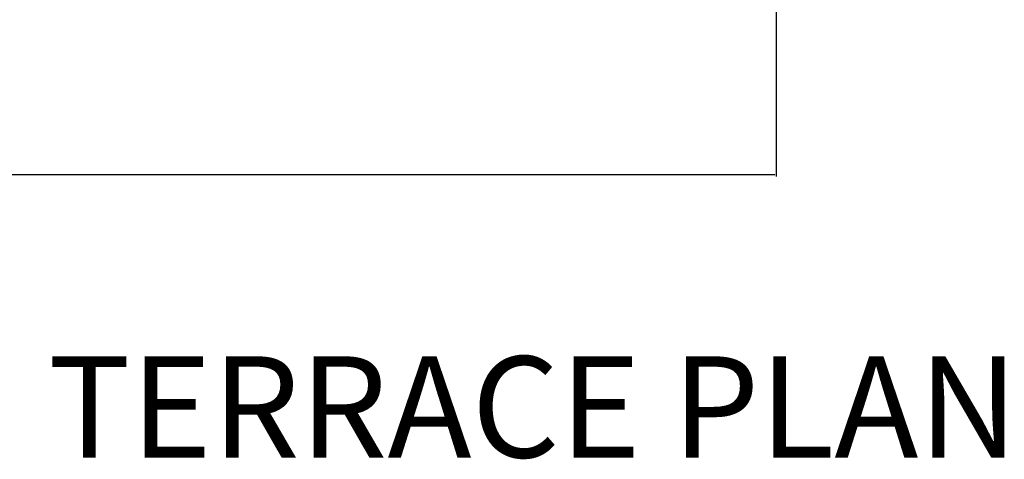
# Model space of a CAD drawing. Units: inches. Extents: x 2166 to 3588, y 1959 to 2628.
# Tile 4 of 13: x 3339 to 3455, y 1964 to 2016. Entities that reach past the tile are written whole.
import ezdxf

# ---------------------------------------------------------------- set-up
doc = ezdxf.new("R2010")
doc.units = ezdxf.units.IN
doc.layers.add('A-ANNO-DIMS', color=2, linetype='Continuous', lineweight=18)
doc.layers.add('A-ANNO-TITL', color=170, linetype='Continuous', lineweight=35)
doc.styles.get("Standard").update_dxf_attribs({"font": 'arial.ttf'})
doc.dimstyles.get("Standard").update_dxf_attribs({"dimtxt": 0.18, "dimasz": 0.18, "dimexe": 0.18, "dimexo": 0.0625, "dimgap": 0.09, "dimtad": 0, "dimtih": 1, "dimtoh": 1, "dimdec": 4, "dimzin": 0, "dimdsep": 46, "dimtxsty": 'Standard', "dimcen": 0.09, "dimadec": 0, "dimazin": 0, "dimtfac": 1, "dimtdec": 4, "dimtofl": 0, "dimtmove": 0, "dimatfit": 3, "dimfxl": 1, "dimtolj": 1, "dimtzin": 0, "dimarcsym": 0})

# ---------------------------------------------------------------- blocks, each defined once
blk = doc.blocks.new('*D50')
at = {"layer": 'A-ANNO-DIMS', "color": 0, "lineweight": -2, "transparency": 16777216}
for p, q in [((3236.47, 2030.92), (3236.47, 1997.05)), ((3428.47, 2030.92), (3428.47, 1997.05)), ((3236.65, 1997.23), (3332.19, 1997.23)), ((3428.29, 1997.23), (3332.75, 1997.23))]:
    blk.add_line(p, q, dxfattribs=at)
at = {"layer": 'A-ANNO-DIMS', "color": 0, "transparency": 16777216}
for points in [[(3236.65, 1997.26), (3236.65, 1997.2), (3236.47, 1997.23)], [(3428.29, 1997.26), (3428.29, 1997.2), (3428.47, 1997.23)]]:
    blk.add_solid(points, dxfattribs=at)
at = {"layer": 'Defpoints', "color": 0, "transparency": 16777216}
for p in [(3236.47, 2030.98), (3428.47, 2030.98), (3428.47, 1997.23)]:
    blk.add_point(p, dxfattribs=at)
at = {"layer": 'A-ANNO-DIMS', "color": 0, "transparency": 16777216, "insert": (3332.47, 1997.23), "char_height": 0.18, "attachment_point": 5}
blk.add_mtext('\\A1;192', dxfattribs=at)

msp = doc.modelspace()

# ---------------------------------------------------------------- texts
at = {"layer": 'A-ANNO-TITL', "insert": (3342.16, 1975.729), "char_height": 12, "attachment_point": 1}
msp.add_mtext_dynamic_manual_height_columns('{\\Fsuperos|c0;TERRACE PLAN }', width=198.49983, gutter_width=12.5, heights=[0], dxfattribs=at)

# ---------------------------------------------------------------- dimensions: what is measured, and where the dimension line sits
at = {"layer": 'A-ANNO-DIMS'}
dim = msp.add_linear_dim(base=(3428.471, 1997.229), p1=(3236.471, 2030.979), p2=(3428.471, 2030.979), dimstyle='Standard', override={"dimdec": 0, "dimlfac": 1, "dimrnd": 0, "dimzin": 0, "dimdsep": 46, "dimlunit": 2}, dxfattribs=at)
dim.commit()
dim.dimension.update_dxf_attribs({"geometry": '*D50', "text_midpoint": (3332.471, 1997.229)})

doc.saveas('drawing.dxf')
